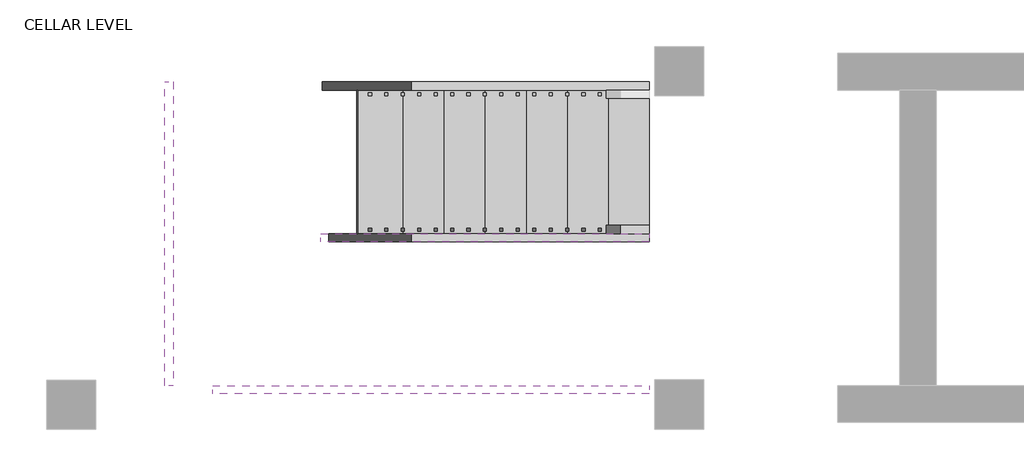
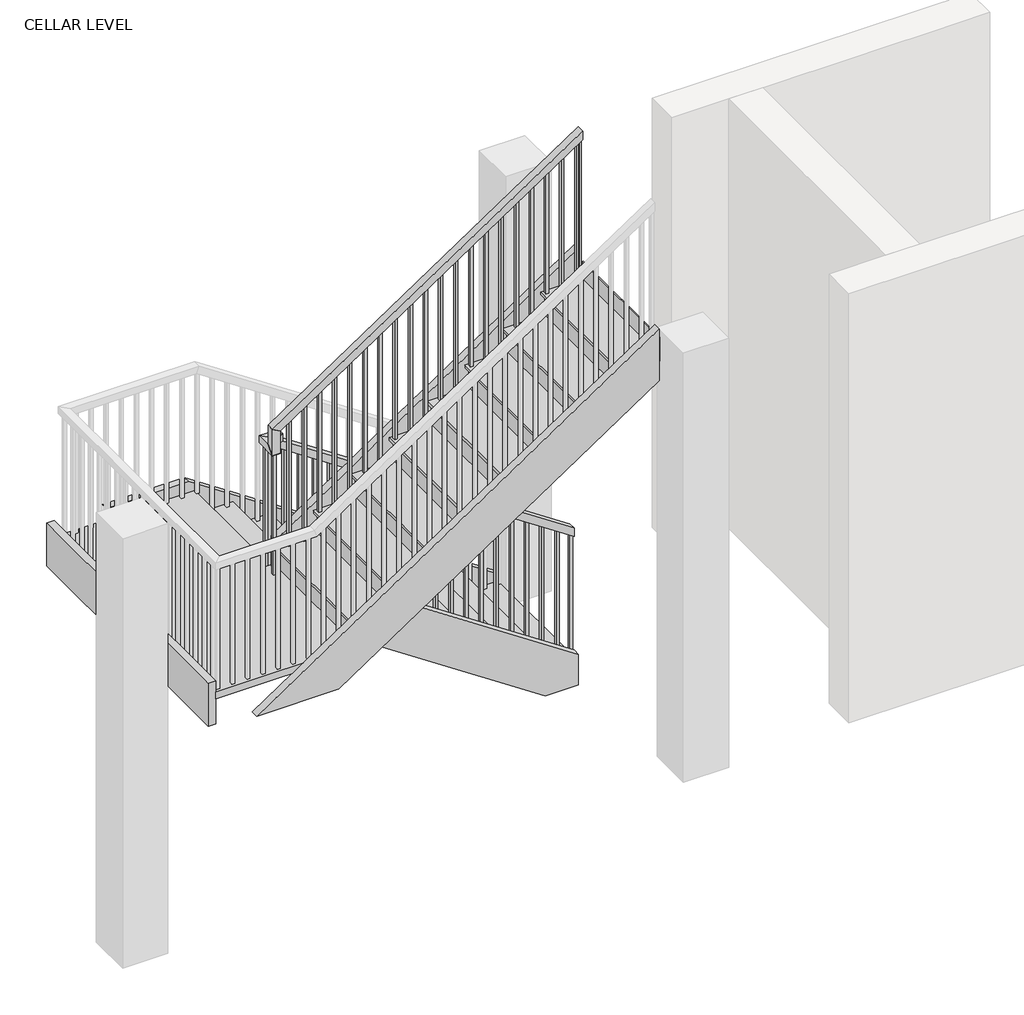
# One storey, part 2 of 2: 5 members, 1 railing, 1 stair flight.
"""IFC4 building model written with IfcOpenShell, lengths in millimetres."""

from ifc_helpers import new_model, si_unit, frame, origin, place, context, project, spatial, polyline, outline, extrude, faceted_brep, transform, mapped, element, save
from components import stair_flight_5a73d723

model = new_model("IFC4")

# Units and contexts
model_context = context("Model", 3, world=origin())
ifc_project = project(units=[si_unit("LENGTHUNIT", "METRE", prefix="MILLI")], contexts=[model_context])

# Site, building, storey
site = spatial("IfcSite", under=ifc_project)
building = spatial("IfcBuilding", under=site)
storey = spatial("IfcBuildingStorey", under=building, Name="CELLAR LEVEL", Elevation=0.0)

# Members
placement = place(None, origin())
element("IfcMember", 1, ObjectType="Stringer - 2\" Width", at=placement, inside=storey, context=model_context, shape_type="SweptSolid", body=[
    extrude(outline(polyline([(0.0, -2748.0012202), (218.0398409, -2748.0012202), (1538.8398409, -4729.2012202), (1172.5158313, -4729.2012202), (0.0, -2970.4274732), (0.0, -2748.0012202)])), frame((0.0, 4990.8309003, 0.0), z_axis=(0.0, 1.0, 0.0), x_axis=(0.0, 0.0, 1.0)), (0.0, 0.0, 1.0), 50.8),
])
element("IfcMember", 2, ObjectType="Stringer - 2\" Width", at=placement, inside=storey, context=model_context, shape_type="SweptSolid", body=[
    extrude(outline(polyline([(1742.0398409, -4780.0012202), (1375.7158313, -4780.0012202), (2730.382498, -2748.0012202), (3096.7065076, -2748.0012202), (1742.0398409, -4780.0012202)])), frame((0.0, 4990.8309003, 0.0), z_axis=(0.0, 1.0, 0.0), x_axis=(0.0, 0.0, 1.0)), (0.0, 0.0, 1.0), 50.8),
])
element("IfcMember", 3, ObjectType="Stringer - 2\" Width", at=placement, inside=storey, context=model_context, shape_type="SweptSolid", body=[
    extrude(outline(polyline([(0.0, -2748.0012202), (218.0398409, -2748.0012202), (1600.2, -4821.2414588), (1600.2, -5370.7274732), (0.0, -2970.4274732), (0.0, -2748.0012202)])), frame((0.0, 5930.6309003, 0.0), z_axis=(0.0, 1.0, 0.0), x_axis=(0.0, 0.0, 1.0)), (0.0, 0.0, 1.0), 50.8),
])
element("IfcMember", 4, ObjectType="Stringer - 2\" Width", at=placement, inside=storey, context=model_context, shape_type="SweptSolid", body=[
    extrude(outline(polyline([(-5745.2012202, 5981.4309003), (-5694.4012202, 5981.4309003), (-5694.4012202, 4101.8309003), (-5745.2012202, 4101.8309003), (-5745.2012202, 5981.4309003)])), frame((0.0, 0.0, 1295.4), z_axis=(0.0, 0.0, 1.0), x_axis=(1.0, 0.0, 0.0)), (0.0, 0.0, 1.0), 304.8),
])
element("IfcMember", 5, ObjectType="Stringer - 2\" Width", at=placement, inside=storey, context=model_context, shape_type="SweptSolid", body=[
    extrude(outline(polyline([(1295.4, -4900.4749672), (2730.382498, -2748.0012202), (3096.7065076, -2748.0012202), (1295.4, -5449.9609815), (1295.4, -4900.4749672)])), frame((0.0, 4051.0309003, 0.0), z_axis=(0.0, 1.0, 0.0), x_axis=(0.0, 0.0, 1.0)), (0.0, 0.0, 1.0), 50.8),
])

# Railing
element("IfcRailing", 6, ObjectType="Handrail - Rectangular", at=placement, inside=storey, context=model_context, shape_type="SolidModel", body=[
    faceted_brep([(-2748.0012202, 5041.6309003, 1083.7333333), (-2748.0012202, 5041.6309003, 1022.6793317), (-2748.0012202, 5092.4309003, 1022.6793317), (-2748.0012202, 5092.4309003, 1083.7333333), (-4703.8012202, 5041.6309003, 2387.6), (-4754.6012202, 5041.6309003, 2360.4126651), (-4754.6012202, 5092.4309003, 2360.4126651), (-4703.8012202, 5092.4309003, 2387.6), (-4703.8012202, 5041.6309003, 2438.4), (-4754.6012202, 5041.6309003, 2387.6), (-4754.6012202, 5092.4309003, 2387.6), (-4703.8012202, 5092.4309003, 2438.4), (-4780.0012202, 5041.6309003, 2438.4), (-4780.0012202, 5041.6309003, 2387.6), (-4830.8012202, 5092.4309003, 2387.6), (-4830.8012202, 5092.4309003, 2438.4), (-4780.0012202, 4990.8309003, 2438.4), (-4830.8012202, 4990.8309003, 2438.4), (-4830.8012202, 4940.0309003, 2387.6), (-4780.0012202, 4940.0309003, 2387.6)], [[[0, 1, 2, 3]], [[1, 0, 4, 5]], [[2, 1, 5, 6]], [[3, 2, 6, 7]], [[0, 3, 7, 4]], [[5, 4, 8, 9]], [[6, 5, 9, 10]], [[7, 6, 10, 11]], [[4, 7, 11, 8]], [[9, 8, 12, 13]], [[10, 9, 13, 14]], [[11, 10, 14, 15]], [[8, 11, 15, 12]], [[16, 17, 18, 19]], [[13, 12, 16, 19]], [[14, 13, 19, 18]], [[15, 14, 18, 17]], [[12, 15, 17, 16]]]),
    faceted_brep([(-4780.0012202, 4990.8309003, 2438.4), (-4780.0012202, 4940.0309003, 2387.6), (-4830.8012202, 4940.0309003, 2387.6), (-4830.8012202, 4990.8309003, 2438.4), (-4780.0012202, 4990.8309003, 2546.6793317), (-4830.8012202, 4990.8309003, 2573.8666667), (-4830.8012202, 4940.0309003, 2573.8666667), (-4780.0012202, 4940.0309003, 2546.6793317)], [[[0, 1, 2, 3]], [[4, 5, 6, 7]], [[1, 0, 4, 7]], [[2, 1, 7, 6]], [[3, 2, 6, 5]], [[0, 3, 5, 4]]]),
    faceted_brep([(-4830.8012202, 4990.8309003, 2573.8666667), (-4780.0012202, 4990.8309003, 2546.6793317), (-4780.0012202, 4940.0309003, 2546.6793317), (-4830.8012202, 4940.0309003, 2573.8666667), (-2748.0012202, 4990.8309003, 3962.4), (-2748.0012202, 4940.0309003, 3962.4), (-2748.0012202, 4940.0309003, 3901.3459984), (-2748.0012202, 4990.8309003, 3901.3459984)], [[[0, 1, 2, 3]], [[4, 5, 6, 7]], [[1, 0, 4, 7]], [[2, 1, 7, 6]], [[3, 2, 6, 5]], [[0, 3, 5, 4]]]),
    extrude(outline(polyline([(3878.0626651, -2782.9262202), (2878.6666667, -2782.9262202), (2878.6666667, -2763.8762202), (3890.7626651, -2763.8762202), (3878.0626651, -2782.9262202)])), frame((0.0, 4955.9059003, 0.0), z_axis=(0.0, 1.0, 0.0), x_axis=(0.0, 0.0, 1.0)), (0.0, 0.0, 1.0), 19.05),
    extrude(outline(polyline([(3810.3293317, -2884.5262202), (2878.6666667, -2884.5262202), (2878.6666667, -2865.4762202), (3823.0293317, -2865.4762202), (3810.3293317, -2884.5262202)])), frame((0.0, 4955.9059003, 0.0), z_axis=(0.0, 1.0, 0.0), x_axis=(0.0, 0.0, 1.0)), (0.0, 0.0, 1.0), 19.05),
    extrude(outline(polyline([(3742.5959984, -2986.1262202), (2878.6666667, -2986.1262202), (2878.6666667, -2967.0762202), (3755.2959984, -2967.0762202), (3742.5959984, -2986.1262202)])), frame((0.0, 4955.9059003, 0.0), z_axis=(0.0, 1.0, 0.0), x_axis=(0.0, 0.0, 1.0)), (0.0, 0.0, 1.0), 19.05),
    extrude(outline(polyline([(3674.8626651, -3087.7262202), (2709.3333333, -3087.7262202), (2709.3333333, -3068.6762202), (3687.5626651, -3068.6762202), (3674.8626651, -3087.7262202)])), frame((0.0, 4955.9059003, 0.0), z_axis=(0.0, 1.0, 0.0), x_axis=(0.0, 0.0, 1.0)), (0.0, 0.0, 1.0), 19.05),
    extrude(outline(polyline([(3607.1293317, -3189.3262202), (2709.3333333, -3189.3262202), (2709.3333333, -3170.2762202), (3619.8293317, -3170.2762202), (3607.1293317, -3189.3262202)])), frame((0.0, 4955.9059003, 0.0), z_axis=(0.0, 1.0, 0.0), x_axis=(0.0, 0.0, 1.0)), (0.0, 0.0, 1.0), 19.05),
    extrude(outline(polyline([(3539.3959984, -3290.9262202), (2540.0, -3290.9262202), (2540.0, -3271.8762202), (3552.0959984, -3271.8762202), (3539.3959984, -3290.9262202)])), frame((0.0, 4955.9059003, 0.0), z_axis=(0.0, 1.0, 0.0), x_axis=(0.0, 0.0, 1.0)), (0.0, 0.0, 1.0), 19.05),
    extrude(outline(polyline([(3471.6626651, -3392.5262202), (2540.0, -3392.5262202), (2540.0, -3373.4762202), (3484.3626651, -3373.4762202), (3471.6626651, -3392.5262202)])), frame((0.0, 4955.9059003, 0.0), z_axis=(0.0, 1.0, 0.0), x_axis=(0.0, 0.0, 1.0)), (0.0, 0.0, 1.0), 19.05),
    extrude(outline(polyline([(3403.9293317, -3494.1262202), (2540.0, -3494.1262202), (2540.0, -3475.0762202), (3416.6293317, -3475.0762202), (3403.9293317, -3494.1262202)])), frame((0.0, 4955.9059003, 0.0), z_axis=(0.0, 1.0, 0.0), x_axis=(0.0, 0.0, 1.0)), (0.0, 0.0, 1.0), 19.05),
    extrude(outline(polyline([(3336.1959984, -3595.7262202), (2370.6666667, -3595.7262202), (2370.6666667, -3576.6762202), (3348.8959984, -3576.6762202), (3336.1959984, -3595.7262202)])), frame((0.0, 4955.9059003, 0.0), z_axis=(0.0, 1.0, 0.0), x_axis=(0.0, 0.0, 1.0)), (0.0, 0.0, 1.0), 19.05),
    extrude(outline(polyline([(3268.4626651, -3697.3262202), (2370.6666667, -3697.3262202), (2370.6666667, -3678.2762202), (3281.1626651, -3678.2762202), (3268.4626651, -3697.3262202)])), frame((0.0, 4955.9059003, 0.0), z_axis=(0.0, 1.0, 0.0), x_axis=(0.0, 0.0, 1.0)), (0.0, 0.0, 1.0), 19.05),
    extrude(outline(polyline([(3200.7293317, -3798.9262202), (2201.3333333, -3798.9262202), (2201.3333333, -3779.8762202), (3213.4293317, -3779.8762202), (3200.7293317, -3798.9262202)])), frame((0.0, 4955.9059003, 0.0), z_axis=(0.0, 1.0, 0.0), x_axis=(0.0, 0.0, 1.0)), (0.0, 0.0, 1.0), 19.05),
    extrude(outline(polyline([(3132.9959984, -3900.5262202), (2201.3333333, -3900.5262202), (2201.3333333, -3881.4762202), (3145.6959984, -3881.4762202), (3132.9959984, -3900.5262202)])), frame((0.0, 4955.9059003, 0.0), z_axis=(0.0, 1.0, 0.0), x_axis=(0.0, 0.0, 1.0)), (0.0, 0.0, 1.0), 19.05),
    extrude(outline(polyline([(3065.2626651, -4002.1262202), (2201.3333333, -4002.1262202), (2201.3333333, -3983.0762202), (3077.9626651, -3983.0762202), (3065.2626651, -4002.1262202)])), frame((0.0, 4955.9059003, 0.0), z_axis=(0.0, 1.0, 0.0), x_axis=(0.0, 0.0, 1.0)), (0.0, 0.0, 1.0), 19.05),
    extrude(outline(polyline([(2997.5293317, -4103.7262202), (2032.0, -4103.7262202), (2032.0, -4084.6762202), (3010.2293317, -4084.6762202), (2997.5293317, -4103.7262202)])), frame((0.0, 4955.9059003, 0.0), z_axis=(0.0, 1.0, 0.0), x_axis=(0.0, 0.0, 1.0)), (0.0, 0.0, 1.0), 19.05),
    extrude(outline(polyline([(2929.7959984, -4205.3262202), (2032.0, -4205.3262202), (2032.0, -4186.2762202), (2942.4959984, -4186.2762202), (2929.7959984, -4205.3262202)])), frame((0.0, 4955.9059003, 0.0), z_axis=(0.0, 1.0, 0.0), x_axis=(0.0, 0.0, 1.0)), (0.0, 0.0, 1.0), 19.05),
    extrude(outline(polyline([(2862.0626651, -4306.9262202), (1862.6666667, -4306.9262202), (1862.6666667, -4287.8762202), (2874.7626651, -4287.8762202), (2862.0626651, -4306.9262202)])), frame((0.0, 4955.9059003, 0.0), z_axis=(0.0, 1.0, 0.0), x_axis=(0.0, 0.0, 1.0)), (0.0, 0.0, 1.0), 19.05),
    extrude(outline(polyline([(2794.3293317, -4408.5262202), (1862.6666667, -4408.5262202), (1862.6666667, -4389.4762202), (2807.0293317, -4389.4762202), (2794.3293317, -4408.5262202)])), frame((0.0, 4955.9059003, 0.0), z_axis=(0.0, 1.0, 0.0), x_axis=(0.0, 0.0, 1.0)), (0.0, 0.0, 1.0), 19.05),
    extrude(outline(polyline([(2726.5959984, -4510.1262202), (1862.6666667, -4510.1262202), (1862.6666667, -4491.0762202), (2739.2959984, -4491.0762202), (2726.5959984, -4510.1262202)])), frame((0.0, 4955.9059003, 0.0), z_axis=(0.0, 1.0, 0.0), x_axis=(0.0, 0.0, 1.0)), (0.0, 0.0, 1.0), 19.05),
    extrude(outline(polyline([(2658.8626651, -4611.7262202), (1693.3333333, -4611.7262202), (1693.3333333, -4592.6762202), (2671.5626651, -4592.6762202), (2658.8626651, -4611.7262202)])), frame((0.0, 4955.9059003, 0.0), z_axis=(0.0, 1.0, 0.0), x_axis=(0.0, 0.0, 1.0)), (0.0, 0.0, 1.0), 19.05),
    extrude(outline(polyline([(2591.1293317, -4713.3262202), (1693.3333333, -4713.3262202), (1693.3333333, -4694.2762202), (2603.8293317, -4694.2762202), (2591.1293317, -4713.3262202)])), frame((0.0, 4955.9059003, 0.0), z_axis=(0.0, 1.0, 0.0), x_axis=(0.0, 0.0, 1.0)), (0.0, 0.0, 1.0), 19.05),
    extrude(outline(polyline([(-4770.4762202, 5057.5059003), (-4789.5262202, 5057.5059003), (-4789.5262202, 5076.5559003), (-4770.4762202, 5076.5559003), (-4770.4762202, 5057.5059003)])), frame((0.0, 0.0, 1524.0), z_axis=(0.0, 0.0, 1.0), x_axis=(1.0, 0.0, 0.0)), (0.0, 0.0, 1.0), 863.6),
    extrude(outline(polyline([(2315.9626651, -4687.9262202), (1354.6666667, -4687.9262202), (1354.6666667, -4668.8762202), (2303.2626651, -4668.8762202), (2315.9626651, -4687.9262202)])), frame((0.0, 5057.5059003, 0.0), z_axis=(0.0, 1.0, 0.0), x_axis=(0.0, 0.0, 1.0)), (0.0, 0.0, 1.0), 19.05),
    extrude(outline(polyline([(2248.2293317, -4586.3262202), (1354.6666667, -4586.3262202), (1354.6666667, -4567.2762202), (2235.5293317, -4567.2762202), (2248.2293317, -4586.3262202)])), frame((0.0, 5057.5059003, 0.0), z_axis=(0.0, 1.0, 0.0), x_axis=(0.0, 0.0, 1.0)), (0.0, 0.0, 1.0), 19.05),
    extrude(outline(polyline([(2180.4959984, -4484.7262202), (1185.3333333, -4484.7262202), (1185.3333333, -4465.6762202), (2167.7959984, -4465.6762202), (2180.4959984, -4484.7262202)])), frame((0.0, 5057.5059003, 0.0), z_axis=(0.0, 1.0, 0.0), x_axis=(0.0, 0.0, 1.0)), (0.0, 0.0, 1.0), 19.05),
    extrude(outline(polyline([(2112.7626651, -4383.1262202), (1185.3333333, -4383.1262202), (1185.3333333, -4364.0762202), (2100.0626651, -4364.0762202), (2112.7626651, -4383.1262202)])), frame((0.0, 5057.5059003, 0.0), z_axis=(0.0, 1.0, 0.0), x_axis=(0.0, 0.0, 1.0)), (0.0, 0.0, 1.0), 19.05),
    extrude(outline(polyline([(2045.0293317, -4281.5262202), (1185.3333333, -4281.5262202), (1185.3333333, -4262.4762202), (2032.3293317, -4262.4762202), (2045.0293317, -4281.5262202)])), frame((0.0, 5057.5059003, 0.0), z_axis=(0.0, 1.0, 0.0), x_axis=(0.0, 0.0, 1.0)), (0.0, 0.0, 1.0), 19.05),
    extrude(outline(polyline([(1977.2959984, -4179.9262202), (1016.0, -4179.9262202), (1016.0, -4160.8762202), (1964.5959984, -4160.8762202), (1977.2959984, -4179.9262202)])), frame((0.0, 5057.5059003, 0.0), z_axis=(0.0, 1.0, 0.0), x_axis=(0.0, 0.0, 1.0)), (0.0, 0.0, 1.0), 19.05),
    extrude(outline(polyline([(1909.5626651, -4078.3262202), (1016.0, -4078.3262202), (1016.0, -4059.2762202), (1896.8626651, -4059.2762202), (1909.5626651, -4078.3262202)])), frame((0.0, 5057.5059003, 0.0), z_axis=(0.0, 1.0, 0.0), x_axis=(0.0, 0.0, 1.0)), (0.0, 0.0, 1.0), 19.05),
    extrude(outline(polyline([(1841.8293317, -3976.7262202), (846.6666667, -3976.7262202), (846.6666667, -3957.6762202), (1829.1293317, -3957.6762202), (1841.8293317, -3976.7262202)])), frame((0.0, 5057.5059003, 0.0), z_axis=(0.0, 1.0, 0.0), x_axis=(0.0, 0.0, 1.0)), (0.0, 0.0, 1.0), 19.05),
    extrude(outline(polyline([(1774.0959984, -3875.1262202), (846.6666667, -3875.1262202), (846.6666667, -3856.0762202), (1761.3959984, -3856.0762202), (1774.0959984, -3875.1262202)])), frame((0.0, 5057.5059003, 0.0), z_axis=(0.0, 1.0, 0.0), x_axis=(0.0, 0.0, 1.0)), (0.0, 0.0, 1.0), 19.05),
    extrude(outline(polyline([(1706.3626651, -3773.5262202), (846.6666667, -3773.5262202), (846.6666667, -3754.4762202), (1693.6626651, -3754.4762202), (1706.3626651, -3773.5262202)])), frame((0.0, 5057.5059003, 0.0), z_axis=(0.0, 1.0, 0.0), x_axis=(0.0, 0.0, 1.0)), (0.0, 0.0, 1.0), 19.05),
    extrude(outline(polyline([(1638.6293317, -3671.9262202), (677.3333333, -3671.9262202), (677.3333333, -3652.8762202), (1625.9293317, -3652.8762202), (1638.6293317, -3671.9262202)])), frame((0.0, 5057.5059003, 0.0), z_axis=(0.0, 1.0, 0.0), x_axis=(0.0, 0.0, 1.0)), (0.0, 0.0, 1.0), 19.05),
    extrude(outline(polyline([(1570.8959984, -3570.3262202), (677.3333333, -3570.3262202), (677.3333333, -3551.2762202), (1558.1959984, -3551.2762202), (1570.8959984, -3570.3262202)])), frame((0.0, 5057.5059003, 0.0), z_axis=(0.0, 1.0, 0.0), x_axis=(0.0, 0.0, 1.0)), (0.0, 0.0, 1.0), 19.05),
    extrude(outline(polyline([(1503.1626651, -3468.7262202), (508.0, -3468.7262202), (508.0, -3449.6762202), (1490.4626651, -3449.6762202), (1503.1626651, -3468.7262202)])), frame((0.0, 5057.5059003, 0.0), z_axis=(0.0, 1.0, 0.0), x_axis=(0.0, 0.0, 1.0)), (0.0, 0.0, 1.0), 19.05),
    extrude(outline(polyline([(1435.4293317, -3367.1262202), (508.0, -3367.1262202), (508.0, -3348.0762202), (1422.7293317, -3348.0762202), (1435.4293317, -3367.1262202)])), frame((0.0, 5057.5059003, 0.0), z_axis=(0.0, 1.0, 0.0), x_axis=(0.0, 0.0, 1.0)), (0.0, 0.0, 1.0), 19.05),
    extrude(outline(polyline([(1367.6959984, -3265.5262202), (508.0, -3265.5262202), (508.0, -3246.4762202), (1354.9959984, -3246.4762202), (1367.6959984, -3265.5262202)])), frame((0.0, 5057.5059003, 0.0), z_axis=(0.0, 1.0, 0.0), x_axis=(0.0, 0.0, 1.0)), (0.0, 0.0, 1.0), 19.05),
    extrude(outline(polyline([(1299.9626651, -3163.9262202), (338.6666667, -3163.9262202), (338.6666667, -3144.8762202), (1287.2626651, -3144.8762202), (1299.9626651, -3163.9262202)])), frame((0.0, 5057.5059003, 0.0), z_axis=(0.0, 1.0, 0.0), x_axis=(0.0, 0.0, 1.0)), (0.0, 0.0, 1.0), 19.05),
    extrude(outline(polyline([(1232.2293317, -3062.3262202), (338.6666667, -3062.3262202), (338.6666667, -3043.2762202), (1219.5293317, -3043.2762202), (1232.2293317, -3062.3262202)])), frame((0.0, 5057.5059003, 0.0), z_axis=(0.0, 1.0, 0.0), x_axis=(0.0, 0.0, 1.0)), (0.0, 0.0, 1.0), 19.05),
    extrude(outline(polyline([(1164.4959984, -2960.7262202), (169.3333333, -2960.7262202), (169.3333333, -2941.6762202), (1151.7959984, -2941.6762202), (1164.4959984, -2960.7262202)])), frame((0.0, 5057.5059003, 0.0), z_axis=(0.0, 1.0, 0.0), x_axis=(0.0, 0.0, 1.0)), (0.0, 0.0, 1.0), 19.05),
    extrude(outline(polyline([(1096.7626651, -2859.1262202), (169.3333333, -2859.1262202), (169.3333333, -2840.0762202), (1084.0626651, -2840.0762202), (1096.7626651, -2859.1262202)])), frame((0.0, 5057.5059003, 0.0), z_axis=(0.0, 1.0, 0.0), x_axis=(0.0, 0.0, 1.0)), (0.0, 0.0, 1.0), 19.05),
    extrude(outline(polyline([(-4795.8762202, 4974.9559003), (-4795.8762202, 4955.9059003), (-4814.9262202, 4955.9059003), (-4814.9262202, 4974.9559003), (-4795.8762202, 4974.9559003)])), frame((0.0, 0.0, 1524.0), z_axis=(0.0, 0.0, 1.0), x_axis=(1.0, 0.0, 0.0)), (0.0, 0.0, 1.0), 863.6),
    extrude(outline(polyline([(-4795.8762202, 5057.5059003), (-4814.9262202, 5057.5059003), (-4814.9262202, 5076.5559003), (-4795.8762202, 5076.5559003), (-4795.8762202, 5057.5059003)])), frame((0.0, 0.0, 1524.0), z_axis=(0.0, 0.0, 1.0), x_axis=(1.0, 0.0, 0.0)), (0.0, 0.0, 1.0), 863.6),
    extrude(outline(polyline([(3888.6459984, -2767.0512202), (2878.6666667, -2767.0512202), (2878.6666667, -2748.0012202), (3901.3459984, -2748.0012202), (3888.6459984, -2767.0512202)])), frame((0.0, 4955.9059003, 0.0), z_axis=(0.0, 1.0, 0.0), x_axis=(0.0, 0.0, 1.0)), (0.0, 0.0, 1.0), 19.05),
    extrude(outline(polyline([(1035.3793317, -2767.0512202), (169.3333333, -2767.0512202), (169.3333333, -2748.0012202), (1022.6793317, -2748.0012202), (1035.3793317, -2767.0512202)])), frame((0.0, 5057.5059003, 0.0), z_axis=(0.0, 1.0, 0.0), x_axis=(0.0, 0.0, 1.0)), (0.0, 0.0, 1.0), 19.05),
])

# Stair flight
stair_flight_shape = stair_flight_5a73d723(model_context)
element("IfcStairFlight", 7, ObjectType="2\" Tread 1\" Nosing 1/4\" Riser", at=placement, inside=storey, context=model_context, shape_type="MappedRepresentation", body=[
    mapped(stair_flight_shape, transform((0.0, 0.0, 0.0), x_axis=(1.0, 0.0, 0.0), y_axis=(0.0, 1.0, 0.0), z_axis=(0.0, 0.0, 1.0))),
])

save(model, "model.ifc")

# Revit data of these elements
# Type "Handrail - Rectangular"
#   Assembly Code = "C2010400"
#   built-in parameter 1008612 = 0.0416667 (stored number, unit not read)
#   built-in parameter 1008611 = 0.0416667 (stored number, unit not read)
#   built-in parameter 1008609 = 0.333333 (stored number, unit not read)
#   built-in parameter 1008604 = 0.166667 (stored number, unit not read)
#   built-in parameter 1008603 = 0.166667 (stored number, unit not read)
#   Railing Height = 3' - 0"
#   built-in parameter 1008630 = 2
#   built-in parameter 1008610 = 2
#   built-in parameter 1008618 = Baluster - Square : 3/4"
# Elements 1, 2, 3, 4, 5 (IfcMember, "Stringer - 2\" Width")
#   Phase Created = New Construction
# Element 6 (IfcRailing, "Handrail - Rectangular")
#   Phase Created = New Construction
# Element 7 (IfcStairFlight, "2\" Tread 1\" Nosing 1/4\" Riser")
#   Phase Created = New Construction
